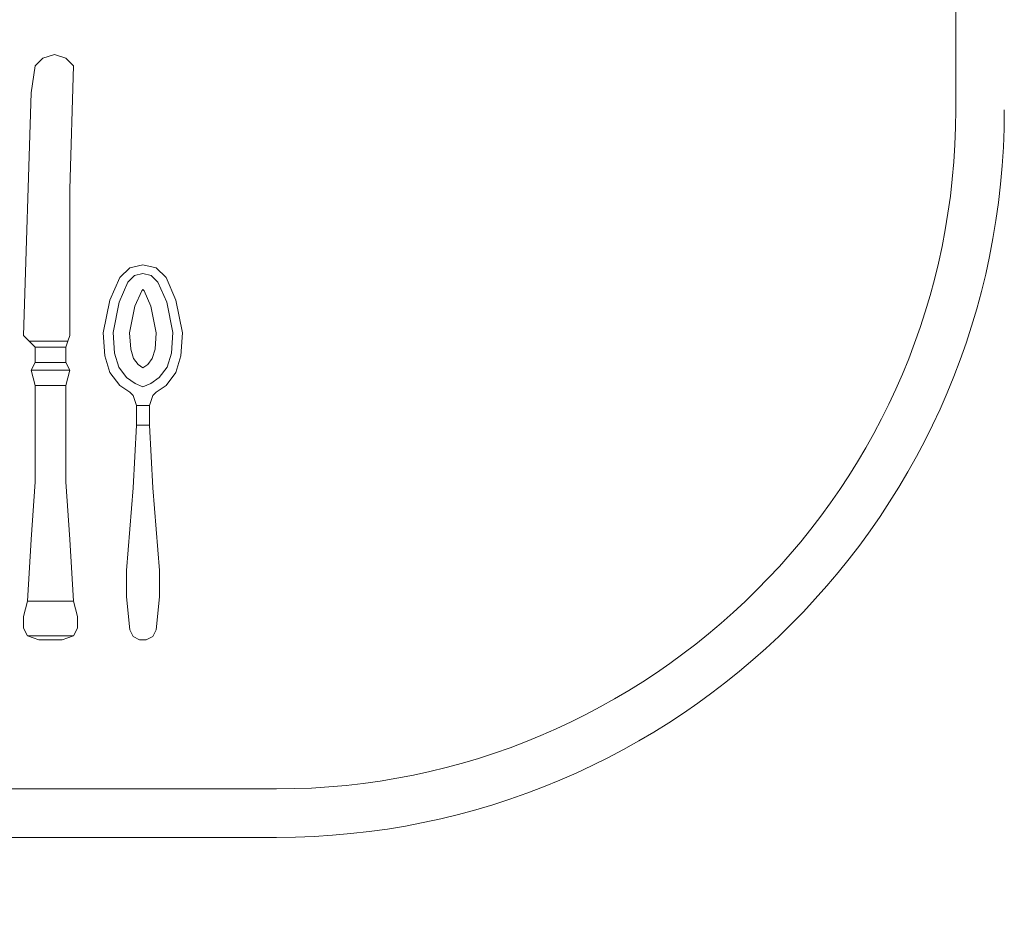
# Model space of a CAD drawing. Units: inches. Extents: x 375 to 1122, y 27 to 1069.
# Tile 105 of 155: x 731.28 to 747.02, y 845.63 to 859.8. Entities that reach past the tile are written whole.
import ezdxf

# ---------------------------------------------------------------- set-up
doc = ezdxf.new("R2010")
doc.units = ezdxf.units.IN
doc.layers.add('A-ANNO-DIMS', color=2, linetype='Continuous', lineweight=18)
doc.layers.add('Furniture', color=30, linetype='Continuous', lineweight=18)
doc.styles.get("Standard").update_dxf_attribs({"font": 'arial.ttf'})
doc.dimstyles.new('ISO-25', dxfattribs={"dimtxt": 12, "dimasz": 2.5, "dimexe": 1.5, "dimexo": 1.5, "dimtad": 1, "dimdec": 1, "dimlunit": 3, "dimtxsty": 'Standard', "dimblk": 'ARCHTICK', "dimcen": 2.5, "dimadec": 0, "dimazin": 0, "dimtfac": 1, "dimtdec": 1, "dimtmove": 0, "dimatfit": 3, "dimfxl": 1.5, "dimfxlon": 1, "dimarcsym": 0})

# ---------------------------------------------------------------- blocks, each defined once
blk = doc.blocks.new('A$C403C54AD')
for p, q in [((0.83575, 1.53256, -0.0006), (1.99923, 1.53256, -0.0006)), ((2.27071, 1.26108, -0.0006), (2.27071, 0.79569, -0.0006)), ((2.2901, 1.26108, -0.0006), (2.2901, 0.79569, -0.0006))]:
    blk.add_line(p, q)
for radius in [0.29087, 0.27148]:
    blk.add_arc((1.99923, 1.26108, -0.0006), radius, 0, 90)
for points, invisible_edges in [([(2.0754, 1.22086, -0.05249), (2.0762, 1.21716, -0.05501), (2.06818, 1.21365, -0.0533), (2.06633, 1.2169, -0.05066)], 5), ([(2.0754, 1.22086, -0.05117), (2.0762, 1.21716, -0.05369), (2.06818, 1.21365, -0.05198), (2.06633, 1.2169, -0.04934)], 5), ([(2.08833, 1.21962, -0.05699), (2.08844, 1.2235, -0.05453), (2.0754, 1.22086, -0.05249), (2.0762, 1.21716, -0.05501)], 5), ([(2.08833, 1.21962, -0.05567), (2.08844, 1.2235, -0.05321), (2.0754, 1.22086, -0.05117), (2.0762, 1.21716, -0.05369)], 5), ([(2.09764, 1.22284, -0.05408), (2.09658, 1.21902, -0.05656), (2.08833, 1.21962, -0.05567), (2.08844, 1.2235, -0.05321)], 5), ([(2.09764, 1.22284, -0.0554), (2.09658, 1.21902, -0.05788), (2.08833, 1.21962, -0.05699), (2.08844, 1.2235, -0.05453)], 5), ([(2.1021, 1.21736, -0.05707), (2.10425, 1.22086, -0.05448), (2.09764, 1.22284, -0.05408), (2.09658, 1.21902, -0.05656)], 5), ([(2.1021, 1.21736, -0.05839), (2.10425, 1.22086, -0.0558), (2.09764, 1.22284, -0.0554), (2.09658, 1.21902, -0.05788)], 5), ([(2.10951, 1.2169, -0.05628), (2.10632, 1.21421, -0.05856), (2.1021, 1.21736, -0.05839), (2.10425, 1.22086, -0.0558)], 5), ([(2.10951, 1.2169, -0.05496), (2.10632, 1.21421, -0.05724), (2.1021, 1.21736, -0.05707), (2.10425, 1.22086, -0.05448)], 5), ([(2.06818, 1.21365, -0.0533), (2.06633, 1.2169, -0.05066), (2.06249, 1.21294, -0.04957), (2.06555, 1.21097, -0.05274)], 5), ([(2.06818, 1.21365, -0.05198), (2.06633, 1.2169, -0.04934), (2.06249, 1.21294, -0.04825), (2.06555, 1.21097, -0.05142)], 5), ([(2.06818, 1.21365, -0.0533), (2.07156, 1.2081, -0.05619), (2.07778, 1.21084, -0.05782), (2.0762, 1.21716, -0.05501)], 5), ([(2.06818, 1.21365, -0.05198), (2.07156, 1.2081, -0.05487), (2.07778, 1.21084, -0.0565), (2.0762, 1.21716, -0.05369)], 5), ([(2.07778, 1.21084, -0.0565), (2.0762, 1.21716, -0.05369), (2.08833, 1.21962, -0.05567), (2.08839, 1.21299, -0.05821)], 5), ([(2.07778, 1.21084, -0.05782), (2.0762, 1.21716, -0.05501), (2.08833, 1.21962, -0.05699), (2.08839, 1.21299, -0.05953)], 5), ([(2.08833, 1.21962, -0.05699), (2.08839, 1.21299, -0.05953), (2.095, 1.21251, -0.06048), (2.09658, 1.21902, -0.05788)], 5), ([(2.08833, 1.21962, -0.05567), (2.08839, 1.21299, -0.05821), (2.095, 1.21251, -0.05916), (2.09658, 1.21902, -0.05656)], 5), ([(2.095, 1.21251, -0.06048), (2.09658, 1.21902, -0.05788), (2.1021, 1.21736, -0.05839), (2.09872, 1.2114, -0.06071)], 5), ([(2.095, 1.21251, -0.05916), (2.09658, 1.21902, -0.05656), (2.1021, 1.21736, -0.05707), (2.09872, 1.2114, -0.05939)], 5), ([(2.1021, 1.21736, -0.05839), (2.09872, 1.2114, -0.06071), (2.1011, 1.20963, -0.06081), (2.10632, 1.21421, -0.05856)], 5), ([(2.1021, 1.21736, -0.05707), (2.09872, 1.2114, -0.05939), (2.1011, 1.20963, -0.05949), (2.10632, 1.21421, -0.05724)], 5), ([(2.10861, 1.2108, -0.05857), (2.11212, 1.21294, -0.05749), (2.10951, 1.2169, -0.05628), (2.10632, 1.21421, -0.05856)], 5), ([(2.10861, 1.2108, -0.05725), (2.11212, 1.21294, -0.05534), (2.10951, 1.2169, -0.05496), (2.10632, 1.21421, -0.05724)], 5), ([(2.06249, 1.21294, -0.04957), (2.06555, 1.21097, -0.05274), (2.06475, 1.20767, -0.05255), (2.06119, 1.20767, -0.04938)], 5), ([(2.06249, 1.21294, -0.04825), (2.06555, 1.21097, -0.05142), (2.06475, 1.20767, -0.05124), (2.06119, 1.20767, -0.04806)], 5), ([(2.07156, 1.2081, -0.05487), (2.06555, 1.21097, -0.05142), (2.06818, 1.21365, -0.05198), (2.07156, 1.2081, -0.05487)], 5), ([(2.07156, 1.2081, -0.05619), (2.06555, 1.21097, -0.05274), (2.06818, 1.21365, -0.0533), (2.07156, 1.2081, -0.05619)], 5), ([(2.07778, 1.21084, -0.0565), (2.07778, 1.20449, -0.0565), (2.08839, 1.20234, -0.05821), (2.08839, 1.21299, -0.05821)], 5), ([(2.07778, 1.21084, -0.05782), (2.07778, 1.20449, -0.05782), (2.08839, 1.20234, -0.05953), (2.08839, 1.21299, -0.05953)], 5), ([(2.08839, 1.20234, -0.05953), (2.08839, 1.21299, -0.05953), (2.095, 1.21251, -0.06048), (2.095, 1.20282, -0.06048)], 5), ([(2.08839, 1.20234, -0.05821), (2.08839, 1.21299, -0.05821), (2.095, 1.21251, -0.05916), (2.095, 1.20282, -0.05916)], 5), ([(2.095, 1.21251, -0.06048), (2.095, 1.20282, -0.06048), (2.09872, 1.20393, -0.06071), (2.09872, 1.2114, -0.06071)], 5), ([(2.095, 1.21251, -0.05916), (2.095, 1.20282, -0.05916), (2.09872, 1.20393, -0.05939), (2.09872, 1.2114, -0.05939)], 5), ([(2.1011, 1.20963, -0.06081), (2.10632, 1.21421, -0.05856), (2.10861, 1.2108, -0.05857), (2.10244, 1.20767, -0.06061)], 5), ([(2.1011, 1.20963, -0.05949), (2.10632, 1.21421, -0.05724), (2.10861, 1.2108, -0.05725), (2.10244, 1.20767, -0.05929)], 5), ([(2.11212, 1.21294, -0.05749), (2.11212, 1.20767, -0.05749), (2.10997, 1.20767, -0.05839), (2.10861, 1.2108, -0.05857)], 11), ([(2.11212, 1.21294, -0.05534), (2.11212, 1.20767, -0.05534), (2.10997, 1.20767, -0.05707), (2.10861, 1.2108, -0.05725)], 11), ([(2.11345, 1.20371, -0.0546), (2.11345, 1.21162, -0.0546), (2.11212, 1.21294, -0.05534), (2.11212, 1.20239, -0.05534)], 5), ([(2.11345, 1.20371, -0.05669), (2.11345, 1.21162, -0.05669), (2.11212, 1.21294, -0.05749), (2.11212, 1.20239, -0.05749)], 5), ([(2.11345, 1.21162, -0.05669), (2.11345, 1.21162, -0.0546), (2.11212, 1.21294, -0.05534), (2.11212, 1.21294, -0.05749)], 1), ([(2.18338, 1.20107, -0.06063), (2.18338, 1.21426, -0.06063), (2.1504, 1.21162, -0.05725), (2.1504, 1.20371, -0.05725)], 5), ([(2.18338, 1.21426, -0.06063), (2.18338, 1.21426, -0.05666), (2.1504, 1.21162, -0.05462), (2.1504, 1.21162, -0.05725)], 4), ([(2.18338, 1.20107, -0.05666), (2.18338, 1.21426, -0.05666), (2.1504, 1.21162, -0.05462), (2.1504, 1.20371, -0.05462)], 5), ([(2.19393, 1.21426, -0.05694), (2.19393, 1.20107, -0.05694), (2.18338, 1.20107, -0.05666), (2.18338, 1.21426, -0.05666)], 5), ([(2.19393, 1.21426, -0.06091), (2.19393, 1.20107, -0.06091), (2.18338, 1.20107, -0.06063), (2.18338, 1.21426, -0.06063)], 5), ([(2.20713, 1.20239, -0.05691), (2.20713, 1.21294, -0.05691), (2.19393, 1.21426, -0.05694), (2.19393, 1.20107, -0.05694)], 5), ([(2.20713, 1.20239, -0.06088), (2.20713, 1.21294, -0.06088), (2.19393, 1.21426, -0.06091), (2.19393, 1.20107, -0.06091)], 5), ([(2.20976, 1.21162, -0.0567), (2.20976, 1.20371, -0.0567), (2.20713, 1.20239, -0.05691), (2.20713, 1.21294, -0.05691)], 5), ([(2.20976, 1.21162, -0.06067), (2.20976, 1.20371, -0.06067), (2.20713, 1.20239, -0.06088), (2.20713, 1.21294, -0.06088)], 5), ([(2.06475, 1.20767, -0.05124), (2.07114, 1.20767, -0.05473), (2.07156, 1.2081, -0.05487), (2.06555, 1.21097, -0.05142)], 5), ([(2.06475, 1.20767, -0.05255), (2.07114, 1.20767, -0.05605), (2.07156, 1.2081, -0.05619), (2.06555, 1.21097, -0.05274)], 5), ([(2.07156, 1.20723, -0.05619), (2.07156, 1.2081, -0.05619), (2.07778, 1.21084, -0.05782), (2.07778, 1.20449, -0.05782)], 5), ([(2.07156, 1.20723, -0.05487), (2.07156, 1.2081, -0.05487), (2.07778, 1.21084, -0.0565), (2.07778, 1.20449, -0.0565)], 5), ([(2.09872, 1.20393, -0.06071), (2.09872, 1.2114, -0.06071), (2.1011, 1.20963, -0.06081), (2.1011, 1.2057, -0.06081)], 5), ([(2.09872, 1.20393, -0.05939), (2.09872, 1.2114, -0.05939), (2.1011, 1.20963, -0.05949), (2.1011, 1.2057, -0.05949)], 5), ([(2.1011, 1.20963, -0.06081), (2.1011, 1.2057, -0.06081), (2.10244, 1.20767, -0.06061)], 1), ([(2.1011, 1.20963, -0.05949), (2.1011, 1.2057, -0.05949), (2.10244, 1.20767, -0.05929)], 1), ([(2.10861, 1.2108, -0.05857), (2.10244, 1.20767, -0.06061), (2.10244, 1.20767, -0.06061), (2.10997, 1.20767, -0.05839)], 5), ([(2.10861, 1.2108, -0.05725), (2.10244, 1.20767, -0.05929), (2.10244, 1.20767, -0.05929), (2.10997, 1.20767, -0.05707)], 5), ([(2.11741, 1.2103, -0.05275), (2.11741, 1.20503, -0.05275), (2.11345, 1.20371, -0.0546), (2.11345, 1.21162, -0.0546)], 4), ([(2.11741, 1.2103, -0.05275), (2.11741, 1.2103, -0.05497), (2.11345, 1.21162, -0.05669), (2.11345, 1.21162, -0.0546)], 5), ([(2.11741, 1.2103, -0.05497), (2.11741, 1.20503, -0.05497), (2.11345, 1.20371, -0.05669), (2.11345, 1.21162, -0.05669)], 4), ([(2.12533, 1.2103, -0.05434), (2.12533, 1.2103, -0.05212), (2.11741, 1.2103, -0.05275), (2.11741, 1.2103, -0.05497)], 5), ([(2.1504, 1.21162, -0.05462), (2.1504, 1.20371, -0.05462), (2.12533, 1.20503, -0.05212), (2.12533, 1.2103, -0.05212)], 1), ([(2.1504, 1.21162, -0.05462), (2.1504, 1.21162, -0.05725), (2.12533, 1.2103, -0.05434), (2.12533, 1.2103, -0.05212)], 5), ([(2.1504, 1.21162, -0.05725), (2.1504, 1.20371, -0.05725), (2.12533, 1.20503, -0.05434), (2.12533, 1.2103, -0.05434)], 1), ([(2.21108, 1.20635, -0.05684), (2.21108, 1.20898, -0.05684), (2.20976, 1.21162, -0.0567), (2.20976, 1.20371, -0.0567)], 4), ([(2.21108, 1.20635, -0.06038), (2.21108, 1.20898, -0.06038), (2.20976, 1.21162, -0.06067), (2.20976, 1.20371, -0.06067)], 4), ([(2.06249, 1.20239, -0.04957), (2.06555, 1.20436, -0.05274), (2.06475, 1.20767, -0.05255), (2.06119, 1.20767, -0.04938)], 5), ([(2.06249, 1.20239, -0.04825), (2.06555, 1.20436, -0.05142), (2.06475, 1.20767, -0.05124), (2.06119, 1.20767, -0.04806)], 5), ([(2.06818, 1.20168, -0.0533), (2.06633, 1.19843, -0.05066), (2.06249, 1.20239, -0.04957), (2.06555, 1.20436, -0.05274)], 5), ([(2.06818, 1.20168, -0.05198), (2.06633, 1.19843, -0.04934), (2.06249, 1.20239, -0.04825), (2.06555, 1.20436, -0.05142)], 5), ([(2.06475, 1.20767, -0.05124), (2.07114, 1.20767, -0.05473), (2.07156, 1.20723, -0.05487), (2.06555, 1.20436, -0.05142)], 5), ([(2.06475, 1.20767, -0.05255), (2.07114, 1.20767, -0.05605), (2.07156, 1.20723, -0.05619), (2.06555, 1.20436, -0.05274)], 5), ([(2.07156, 1.20723, -0.05487), (2.06555, 1.20436, -0.05142), (2.06818, 1.20168, -0.05198), (2.07156, 1.20723, -0.05487)], 5), ([(2.07156, 1.20723, -0.05619), (2.06555, 1.20436, -0.05274), (2.06818, 1.20168, -0.0533), (2.07156, 1.20723, -0.05619)], 5), ([(2.06818, 1.20168, -0.0533), (2.07156, 1.20723, -0.05619), (2.07778, 1.20449, -0.05782), (2.0762, 1.19817, -0.05501)], 5), ([(2.06818, 1.20168, -0.05198), (2.07156, 1.20723, -0.05487), (2.07778, 1.20449, -0.0565), (2.0762, 1.19817, -0.05369)], 5), ([(2.07114, 1.20767, -0.05473), (2.07156, 1.2081, -0.05487), (2.07156, 1.20723, -0.05487), (2.07114, 1.20767, -0.05473)], 2), ([(2.07114, 1.20767, -0.05605), (2.07156, 1.2081, -0.05619), (2.07156, 1.20723, -0.05619), (2.07114, 1.20767, -0.05605)], 2), ([(2.07778, 1.20449, -0.0565), (2.0762, 1.19817, -0.05369), (2.08833, 1.19571, -0.05567), (2.08839, 1.20234, -0.05821)], 5), ([(2.07778, 1.20449, -0.05782), (2.0762, 1.19817, -0.05501), (2.08833, 1.19571, -0.05699), (2.08839, 1.20234, -0.05953)], 5), ([(2.1021, 1.19797, -0.05839), (2.09872, 1.20393, -0.06071), (2.1011, 1.2057, -0.06081), (2.10632, 1.20112, -0.05856)], 5), ([(2.1021, 1.19797, -0.05707), (2.09872, 1.20393, -0.05939), (2.1011, 1.2057, -0.05949), (2.10632, 1.20112, -0.05724)], 5), ([(2.1011, 1.2057, -0.06081), (2.10632, 1.20112, -0.05856), (2.10861, 1.20453, -0.05857), (2.10244, 1.20767, -0.06061)], 5), ([(2.1011, 1.2057, -0.05949), (2.10632, 1.20112, -0.05724), (2.10861, 1.20453, -0.05725), (2.10244, 1.20767, -0.05929)], 5), ([(2.10861, 1.20453, -0.05857), (2.10244, 1.20767, -0.06061), (2.10244, 1.20767, -0.06061), (2.10997, 1.20767, -0.05839)], 5), ([(2.10861, 1.20453, -0.05725), (2.10244, 1.20767, -0.05929), (2.10244, 1.20767, -0.05929), (2.10997, 1.20767, -0.05707)], 5), ([(2.10861, 1.20453, -0.05725), (2.11212, 1.20239, -0.05534), (2.10951, 1.19843, -0.05496), (2.10632, 1.20112, -0.05724)], 5), ([(2.11212, 1.20239, -0.05749), (2.11212, 1.20767, -0.05749), (2.10997, 1.20767, -0.05839), (2.10861, 1.20453, -0.05857)], 11), ([(2.11212, 1.20239, -0.05534), (2.11212, 1.20767, -0.05534), (2.10997, 1.20767, -0.05707), (2.10861, 1.20453, -0.05725)], 11), ([(2.11741, 1.20503, -0.05497), (2.11741, 1.20503, -0.05275), (2.11345, 1.20371, -0.0546), (2.11345, 1.20371, -0.05669)], 5), ([(2.11741, 1.20503, -0.05497), (2.11741, 1.20503, -0.05275), (2.12533, 1.20503, -0.05212), (2.12533, 1.20503, -0.05434)], 5), ([(2.12533, 1.20503, -0.05212), (2.12533, 1.20503, -0.05434), (2.1504, 1.20371, -0.05725), (2.1504, 1.20371, -0.05462)], 5), ([(2.0754, 1.19447, -0.05249), (2.0762, 1.19817, -0.05501), (2.06818, 1.20168, -0.0533), (2.06633, 1.19843, -0.05066)], 5), ([(2.0754, 1.19447, -0.05117), (2.0762, 1.19817, -0.05369), (2.06818, 1.20168, -0.05198), (2.06633, 1.19843, -0.04934)], 5), ([(2.08833, 1.19571, -0.05699), (2.08839, 1.20234, -0.05953), (2.095, 1.20282, -0.06048), (2.09658, 1.19631, -0.05788)], 5), ([(2.08833, 1.19571, -0.05567), (2.08839, 1.20234, -0.05821), (2.095, 1.20282, -0.05916), (2.09658, 1.19631, -0.05656)], 5), ([(2.095, 1.20282, -0.05916), (2.09658, 1.19631, -0.05656), (2.1021, 1.19797, -0.05707), (2.09872, 1.20393, -0.05939)], 5), ([(2.10951, 1.19843, -0.05628), (2.10632, 1.20112, -0.05856), (2.1021, 1.19797, -0.05839), (2.10425, 1.19447, -0.0558)], 5), ([(2.10951, 1.19843, -0.05496), (2.10632, 1.20112, -0.05724), (2.1021, 1.19797, -0.05707), (2.10425, 1.19447, -0.05448)], 5), ([(2.11345, 1.20371, -0.0546), (2.11345, 1.20371, -0.05669), (2.11212, 1.20239, -0.05749), (2.11212, 1.20239, -0.05534)], 1), ([(2.1504, 1.20371, -0.05725), (2.1504, 1.20371, -0.05462), (2.18338, 1.20107, -0.05666), (2.18338, 1.20107, -0.06063)], 1), ([(2.08833, 1.19571, -0.05699), (2.08844, 1.19183, -0.05453), (2.0754, 1.19447, -0.05249), (2.0762, 1.19817, -0.05501)], 5), ([(2.08833, 1.19571, -0.05567), (2.08844, 1.19183, -0.05321), (2.0754, 1.19447, -0.05117), (2.0762, 1.19817, -0.05369)], 5), ([(2.1021, 1.19797, -0.05707), (2.10425, 1.19447, -0.05448), (2.09764, 1.19249, -0.05408), (2.09658, 1.19631, -0.05656)], 5), ([(2.1021, 1.19797, -0.05839), (2.10425, 1.19447, -0.0558), (2.09764, 1.19249, -0.0554), (2.09658, 1.19631, -0.05788)], 5), ([(2.09764, 1.19249, -0.05408), (2.09658, 1.19631, -0.05656), (2.08833, 1.19571, -0.05567), (2.08844, 1.19183, -0.05321)], 5), ([(2.09764, 1.19249, -0.0554), (2.09658, 1.19631, -0.05788), (2.08833, 1.19571, -0.05699), (2.08844, 1.19183, -0.05453)], 5), ([(2.19569, 1.17996, -0.05014), (2.19569, 1.16149, -0.05014), (2.20185, 1.15995, -0.0486), (2.20185, 1.1815, -0.0486)], 4), ([(2.19569, 1.17996, -0.05938), (2.19569, 1.16149, -0.05938), (2.20185, 1.15995, -0.06091), (2.20185, 1.1815, -0.06091)], 4), ([(2.20185, 1.15995, -0.0486), (2.20185, 1.1815, -0.0486), (2.20647, 1.1815, -0.05014), (2.20647, 1.15995, -0.05014)], 5), ([(2.20185, 1.15995, -0.06091), (2.20185, 1.1815, -0.06091), (2.20647, 1.1815, -0.05938), (2.20647, 1.15995, -0.05938)], 5), ([(2.20647, 1.1815, -0.05014), (2.20647, 1.15995, -0.05014), (2.20954, 1.16149, -0.05168), (2.20954, 1.17996, -0.05168)], 1), ([(2.20647, 1.1815, -0.05938), (2.20647, 1.15995, -0.05938), (2.20954, 1.16149, -0.05784), (2.20954, 1.17996, -0.05784)], 1), ([(1.97713, 1.17226, -0.05399), (1.97713, 1.17226, -0.05399), (1.97867, 1.17688, -0.05399), (1.97867, 1.16765, -0.05399)], 4), ([(1.97713, 1.17226, -0.05553), (1.97713, 1.17226, -0.05553), (1.97867, 1.17688, -0.05553), (1.97867, 1.16765, -0.05553)], 4), ([(1.97867, 1.17688, -0.05553), (1.97867, 1.17688, -0.05399), (1.97713, 1.17226, -0.05399), (1.97713, 1.17226, -0.05553)], 1), ([(1.97867, 1.17688, -0.05399), (1.97867, 1.16765, -0.05399), (1.98174, 1.16457, -0.05399), (1.98174, 1.17996, -0.05399)], 5), ([(1.97867, 1.17688, -0.05553), (1.97867, 1.16765, -0.05553), (1.98174, 1.16457, -0.05553), (1.98174, 1.17996, -0.05553)], 5), ([(1.98174, 1.17996, -0.05399), (1.98174, 1.17996, -0.05553), (1.97867, 1.17688, -0.05553), (1.97867, 1.17688, -0.05399)], 5), ([(1.98174, 1.16457, -0.05399), (1.98174, 1.17996, -0.05399), (2.031, 1.17842, -0.05399), (1.99252, 1.16303, -0.05399)], 5), ([(1.98174, 1.16457, -0.05553), (1.98174, 1.17996, -0.05553), (2.031, 1.17842, -0.05553), (1.99252, 1.16303, -0.05553)], 5), ([(2.031, 1.17842, -0.05553), (2.031, 1.17842, -0.05399), (1.98174, 1.17996, -0.05399), (1.98174, 1.17996, -0.05553)], 5), ([(2.031, 1.17842, -0.05399), (1.99252, 1.16303, -0.05399), (2.08949, 1.15995, -0.05399), (2.08949, 1.17842, -0.05399)], 5), ([(2.031, 1.17842, -0.05553), (1.99252, 1.16303, -0.05553), (2.08949, 1.15995, -0.05553), (2.08949, 1.17842, -0.05553)], 5), ([(2.08949, 1.17842, -0.05399), (2.08949, 1.17842, -0.05553), (2.031, 1.17842, -0.05553), (2.031, 1.17842, -0.05399)], 5), ([(2.08949, 1.15995, -0.05399), (2.08949, 1.17842, -0.05399), (2.0918, 1.17765, -0.05322), (2.0918, 1.16226, -0.05322)], 1), ([(2.08949, 1.15995, -0.05553), (2.08949, 1.17842, -0.05553), (2.0918, 1.17765, -0.0563), (2.0918, 1.16226, -0.0563)], 1), ([(2.0918, 1.17765, -0.0563), (2.0918, 1.17765, -0.05322), (2.08949, 1.17842, -0.05399), (2.08949, 1.17842, -0.05553)], 5), ([(2.0941, 1.17688, -0.05014), (2.0941, 1.17688, -0.05938), (2.0918, 1.17765, -0.0563), (2.0918, 1.17765, -0.05322)], 5), ([(2.10026, 1.17688, -0.05938), (2.10026, 1.17688, -0.05014), (2.0941, 1.17688, -0.05014), (2.0941, 1.17688, -0.05938)], 4), ([(2.1095, 1.16457, -0.05014), (2.1095, 1.17688, -0.05014), (2.14798, 1.17688, -0.0486), (2.14798, 1.16457, -0.0486)], 4), ([(2.1095, 1.16457, -0.05938), (2.1095, 1.17688, -0.05938), (2.14798, 1.17688, -0.06091), (2.14798, 1.16457, -0.06091)], 4), ([(2.14798, 1.17688, -0.0486), (2.14798, 1.16457, -0.0486), (2.17106, 1.16303, -0.0486), (2.17106, 1.17842, -0.0486)], 5), ([(2.14798, 1.17688, -0.06091), (2.14798, 1.16457, -0.06091), (2.17106, 1.16303, -0.06091), (2.17106, 1.17842, -0.06091)], 5), ([(2.17106, 1.16303, -0.0486), (2.17106, 1.17842, -0.0486), (2.19569, 1.17996, -0.05014), (2.19569, 1.16149, -0.05014)], 1), ([(2.17106, 1.16303, -0.06091), (2.17106, 1.17842, -0.06091), (2.19569, 1.17996, -0.05938), (2.19569, 1.16149, -0.05938)], 1), ([(1.97713, 1.17226, -0.05399), (1.97713, 1.17226, -0.05553), (1.97867, 1.16765, -0.05553), (1.97867, 1.16765, -0.05399)], 4), ([(1.97867, 1.16765, -0.05553), (1.97867, 1.16765, -0.05399), (1.98174, 1.16457, -0.05399), (1.98174, 1.16457, -0.05553)], 5), ([(1.98174, 1.16457, -0.05399), (1.98174, 1.16457, -0.05553), (1.99252, 1.16303, -0.05553), (1.99252, 1.16303, -0.05399)], 5), ([(1.99252, 1.16303, -0.05553), (1.99252, 1.16303, -0.05399), (2.08949, 1.15995, -0.05399), (2.08949, 1.15995, -0.05553)], 5), ([(2.08949, 1.15995, -0.05553), (2.08949, 1.15995, -0.05399), (2.0918, 1.16226, -0.05322), (2.0918, 1.16226, -0.0563)], 5), ([(2.0918, 1.16226, -0.05322), (2.0918, 1.16226, -0.0563), (2.0941, 1.16457, -0.05938), (2.0941, 1.16457, -0.05014)], 5), ([(2.0941, 1.16457, -0.05938), (2.0941, 1.16457, -0.05014), (2.10026, 1.16457, -0.05014), (2.10026, 1.16457, -0.05938)], 1)]:
    blk.add_3dface(points, dxfattribs=dict(invisible_edges=invisible_edges))
for points in [[(2.0754, 1.22086, -0.05117), (2.0754, 1.22086, -0.05249), (2.06633, 1.2169, -0.05066), (2.06633, 1.2169, -0.04934)], [(2.08844, 1.2235, -0.05453), (2.08844, 1.2235, -0.05321), (2.0754, 1.22086, -0.05117), (2.0754, 1.22086, -0.05249)], [(2.09764, 1.22284, -0.05408), (2.09764, 1.22284, -0.0554), (2.08844, 1.2235, -0.05453), (2.08844, 1.2235, -0.05321)], [(2.10425, 1.22086, -0.0558), (2.10425, 1.22086, -0.05448), (2.09764, 1.22284, -0.05408), (2.09764, 1.22284, -0.0554)], [(2.10951, 1.2169, -0.05496), (2.10951, 1.2169, -0.05628), (2.10425, 1.22086, -0.0558), (2.10425, 1.22086, -0.05448)], [(2.06633, 1.2169, -0.05066), (2.06633, 1.2169, -0.04934), (2.06249, 1.21294, -0.04825), (2.06249, 1.21294, -0.04957)], [(2.11212, 1.21294, -0.05749), (2.11212, 1.21294, -0.05534), (2.10951, 1.2169, -0.05496), (2.10951, 1.2169, -0.05628)], [(2.06249, 1.21294, -0.04825), (2.06249, 1.21294, -0.04957), (2.06119, 1.20767, -0.04938), (2.06119, 1.20767, -0.04806)], [(2.19393, 1.21426, -0.05694), (2.19393, 1.21426, -0.06091), (2.18338, 1.21426, -0.06063), (2.18338, 1.21426, -0.05666)], [(2.20713, 1.21294, -0.06088), (2.20713, 1.21294, -0.05691), (2.19393, 1.21426, -0.05694), (2.19393, 1.21426, -0.06091)], [(2.20976, 1.21162, -0.0567), (2.20976, 1.21162, -0.06067), (2.20713, 1.21294, -0.06088), (2.20713, 1.21294, -0.05691)], [(2.12533, 1.20503, -0.05434), (2.12533, 1.2103, -0.05434), (2.11741, 1.2103, -0.05497), (2.11741, 1.20503, -0.05497)], [(2.12533, 1.20503, -0.05212), (2.12533, 1.2103, -0.05212), (2.11741, 1.2103, -0.05275), (2.11741, 1.20503, -0.05275)], [(2.21108, 1.20898, -0.06038), (2.21108, 1.20898, -0.05684), (2.20976, 1.21162, -0.0567), (2.20976, 1.21162, -0.06067)], [(2.21108, 1.20635, -0.05684), (2.21108, 1.20635, -0.06038), (2.21108, 1.20898, -0.06038), (2.21108, 1.20898, -0.05684)], [(2.06119, 1.20767, -0.04938), (2.06119, 1.20767, -0.04806), (2.06249, 1.20239, -0.04825), (2.06249, 1.20239, -0.04957)], [(2.20976, 1.20371, -0.06067), (2.20976, 1.20371, -0.0567), (2.21108, 1.20635, -0.05684), (2.21108, 1.20635, -0.06038)], [(2.06249, 1.20239, -0.04825), (2.06249, 1.20239, -0.04957), (2.06633, 1.19843, -0.05066), (2.06633, 1.19843, -0.04934)], [(2.10951, 1.19843, -0.05628), (2.10951, 1.19843, -0.05496), (2.11212, 1.20239, -0.05534), (2.11212, 1.20239, -0.05749)], [(2.18338, 1.20107, -0.05666), (2.18338, 1.20107, -0.06063), (2.19393, 1.20107, -0.06091), (2.19393, 1.20107, -0.05694)], [(2.19393, 1.20107, -0.06091), (2.19393, 1.20107, -0.05694), (2.20713, 1.20239, -0.05691), (2.20713, 1.20239, -0.06088)], [(2.20713, 1.20239, -0.05691), (2.20713, 1.20239, -0.06088), (2.20976, 1.20371, -0.06067), (2.20976, 1.20371, -0.0567)], [(2.06633, 1.19843, -0.05066), (2.06633, 1.19843, -0.04934), (2.0754, 1.19447, -0.05117), (2.0754, 1.19447, -0.05249)], [(2.10425, 1.19447, -0.05448), (2.10425, 1.19447, -0.0558), (2.10951, 1.19843, -0.05628), (2.10951, 1.19843, -0.05496)], [(2.0754, 1.19447, -0.05117), (2.0754, 1.19447, -0.05249), (2.08844, 1.19183, -0.05453), (2.08844, 1.19183, -0.05321)], [(2.08844, 1.19183, -0.05453), (2.08844, 1.19183, -0.05321), (2.09764, 1.19249, -0.05408), (2.09764, 1.19249, -0.0554)], [(2.09764, 1.19249, -0.0554), (2.09764, 1.19249, -0.05408), (2.10425, 1.19447, -0.05448), (2.10425, 1.19447, -0.0558)], [(2.20185, 1.1815, -0.06091), (2.20185, 1.1815, -0.0486), (2.19569, 1.17996, -0.05014), (2.19569, 1.17996, -0.05938)], [(2.20647, 1.1815, -0.05014), (2.20647, 1.1815, -0.05938), (2.20185, 1.1815, -0.06091), (2.20185, 1.1815, -0.0486)], [(2.20954, 1.17996, -0.05168), (2.20954, 1.17996, -0.05784), (2.20647, 1.1815, -0.05938), (2.20647, 1.1815, -0.05014)], [(2.0918, 1.16226, -0.05322), (2.0918, 1.17765, -0.05322), (2.0941, 1.17688, -0.05014), (2.0941, 1.16457, -0.05014)], [(2.0918, 1.16226, -0.0563), (2.0918, 1.17765, -0.0563), (2.0941, 1.17688, -0.05938), (2.0941, 1.16457, -0.05938)], [(2.0941, 1.17688, -0.05014), (2.0941, 1.16457, -0.05014), (2.10026, 1.16457, -0.05014), (2.10026, 1.17688, -0.05014)], [(2.0941, 1.17688, -0.05938), (2.0941, 1.16457, -0.05938), (2.10026, 1.16457, -0.05938), (2.10026, 1.17688, -0.05938)], [(2.10026, 1.16457, -0.05014), (2.10026, 1.17688, -0.05014), (2.10334, 1.17842, -0.0486), (2.10334, 1.16303, -0.0486)], [(2.10026, 1.16457, -0.05938), (2.10026, 1.17688, -0.05938), (2.10334, 1.17842, -0.06091), (2.10334, 1.16303, -0.06091)], [(2.10334, 1.17842, -0.0486), (2.10334, 1.17842, -0.06091), (2.10026, 1.17688, -0.05938), (2.10026, 1.17688, -0.05014)], [(2.10334, 1.17842, -0.0486), (2.10334, 1.16303, -0.0486), (2.1095, 1.16457, -0.05014), (2.1095, 1.17688, -0.05014)], [(2.10334, 1.17842, -0.06091), (2.10334, 1.16303, -0.06091), (2.1095, 1.16457, -0.05938), (2.1095, 1.17688, -0.05938)], [(2.1095, 1.17688, -0.05938), (2.1095, 1.17688, -0.05014), (2.10334, 1.17842, -0.0486), (2.10334, 1.17842, -0.06091)], [(2.14798, 1.17688, -0.0486), (2.14798, 1.17688, -0.06091), (2.1095, 1.17688, -0.05938), (2.1095, 1.17688, -0.05014)], [(2.17106, 1.17842, -0.06091), (2.17106, 1.17842, -0.0486), (2.14798, 1.17688, -0.0486), (2.14798, 1.17688, -0.06091)], [(2.19569, 1.17996, -0.05014), (2.19569, 1.17996, -0.05938), (2.17106, 1.17842, -0.06091), (2.17106, 1.17842, -0.0486)], [(2.20954, 1.16149, -0.05168), (2.20954, 1.17996, -0.05168), (2.21108, 1.17534, -0.05476), (2.21108, 1.16611, -0.05476)], [(2.21108, 1.17534, -0.05476), (2.21108, 1.17534, -0.05476), (2.20954, 1.17996, -0.05168), (2.20954, 1.17996, -0.05784)], [(2.20954, 1.16149, -0.05784), (2.20954, 1.17996, -0.05784), (2.21108, 1.17534, -0.05476), (2.21108, 1.16611, -0.05476)], [(2.20954, 1.16149, -0.05168), (2.20954, 1.16149, -0.05784), (2.21108, 1.16611, -0.05476)], [(2.10026, 1.16457, -0.05014), (2.10026, 1.16457, -0.05938), (2.10334, 1.16303, -0.06091), (2.10334, 1.16303, -0.0486)], [(2.10334, 1.16303, -0.06091), (2.10334, 1.16303, -0.0486), (2.1095, 1.16457, -0.05014), (2.1095, 1.16457, -0.05938)], [(2.1095, 1.16457, -0.05014), (2.1095, 1.16457, -0.05938), (2.14798, 1.16457, -0.06091), (2.14798, 1.16457, -0.0486)], [(2.14798, 1.16457, -0.06091), (2.14798, 1.16457, -0.0486), (2.17106, 1.16303, -0.0486), (2.17106, 1.16303, -0.06091)], [(2.17106, 1.16303, -0.0486), (2.17106, 1.16303, -0.06091), (2.19569, 1.16149, -0.05938), (2.19569, 1.16149, -0.05014)], [(2.19569, 1.16149, -0.05938), (2.19569, 1.16149, -0.05014), (2.20185, 1.15995, -0.0486), (2.20185, 1.15995, -0.06091)], [(2.20647, 1.15995, -0.05938), (2.20647, 1.15995, -0.05014), (2.20954, 1.16149, -0.05168), (2.20954, 1.16149, -0.05784)], [(2.20185, 1.15995, -0.0486), (2.20185, 1.15995, -0.06091), (2.20647, 1.15995, -0.05938), (2.20647, 1.15995, -0.05014)]]:
    blk.add_3dface(points)
blk = doc.blocks.new('_ArchTick')
at = {"color": 0, "linetype": 'ByBlock', "const_width": 0.15}
blk.add_lwpolyline([(-0.5, -0.5), (0.5, 0.5)], dxfattribs=at)
blk = doc.blocks.new('*D85')
at = {"layer": 'A-ANNO-DIMS', "color": 0, "lineweight": -2, "transparency": 16777216}
for p, q in [((401.507, 868.528), (398.507, 868.528)), ((400.007, 814.528), (400.007, 868.528)), ((401.507, 814.528), (398.507, 814.528))]:
    blk.add_line(p, q, dxfattribs=at)
at = {"layer": 'Defpoints', "color": 0, "transparency": 16777216}
for p in [(400.007, 868.528), (845.007, 868.528), (845.007, 814.528)]:
    blk.add_point(p, dxfattribs=at)
at = {"layer": 'A-ANNO-DIMS', "color": 0, "lineweight": -2, "transparency": 16777216, "xscale": 2.5, "yscale": 2.5, "zscale": 2.5}
for p, rotation in [((400.007, 868.528), 90), ((400.007, 814.528), 270)]:
    blk.add_blockref('_ArchTick', p, dxfattribs=dict(at, rotation=rotation))
at = {"layer": 'A-ANNO-DIMS', "color": 0, "transparency": 16777216, "insert": (393.255, 841.528), "char_height": 12, "attachment_point": 5, "rotation": 90}
blk.add_mtext('4\'-6"', dxfattribs=at)
blk = doc.blocks.new('*D88')
at = {"layer": 'A-ANNO-DIMS', "color": 0, "lineweight": -2, "transparency": 16777216}
for p, q in [((731.007, 1052.528), (731.007, 1055.528)), ((854.007, 1052.528), (854.007, 1055.528)), ((731.007, 1054.028), (854.007, 1054.028))]:
    blk.add_line(p, q, dxfattribs=at)
at = {"layer": 'Defpoints', "color": 0, "transparency": 16777216}
for p in [(854.007, 1054.028), (731.007, 502.528), (854.007, 502.528)]:
    blk.add_point(p, dxfattribs=at)
at = {"layer": 'A-ANNO-DIMS', "color": 0, "lineweight": -2, "transparency": 16777216, "xscale": 2.5, "yscale": 2.5, "zscale": 2.5, "rotation": 180}
blk.add_blockref('_ArchTick', (731.007, 1054.028), dxfattribs=at)
at = {"layer": 'A-ANNO-DIMS', "color": 0, "lineweight": -2, "transparency": 16777216, "xscale": 2.5, "yscale": 2.5, "zscale": 2.5}
blk.add_blockref('_ArchTick', (854.007, 1054.028), dxfattribs=at)
at = {"layer": 'A-ANNO-DIMS', "color": 0, "transparency": 16777216, "insert": (792.507, 1060.784), "char_height": 12, "attachment_point": 5}
blk.add_mtext('10\'-3"', dxfattribs=at)
blk = doc.blocks.new('*D91')
at = {"layer": 'A-ANNO-DIMS', "color": 0, "lineweight": -2, "transparency": 16777216}
for p, q in [((728.007, 1052.528), (728.007, 1055.528)), ((788.007, 1052.528), (788.007, 1055.528)), ((728.007, 1054.028), (788.007, 1054.028))]:
    blk.add_line(p, q, dxfattribs=at)
at = {"layer": 'Defpoints', "color": 0, "transparency": 16777216}
for p in [(788.007, 1054.028), (728.007, 774.028), (788.007, 774.028)]:
    blk.add_point(p, dxfattribs=at)
at = {"layer": 'A-ANNO-DIMS', "color": 0, "lineweight": -2, "transparency": 16777216, "xscale": 2.5, "yscale": 2.5, "zscale": 2.5, "rotation": 180}
blk.add_blockref('_ArchTick', (728.007, 1054.028), dxfattribs=at)
at = {"layer": 'A-ANNO-DIMS', "color": 0, "lineweight": -2, "transparency": 16777216, "xscale": 2.5, "yscale": 2.5, "zscale": 2.5}
blk.add_blockref('_ArchTick', (788.007, 1054.028), dxfattribs=at)
at = {"layer": 'A-ANNO-DIMS', "color": 0, "transparency": 16777216, "insert": (758.007, 1060.78), "char_height": 12, "attachment_point": 5}
blk.add_mtext('5\'-0"', dxfattribs=at)

msp = doc.modelspace()

# ---------------------------------------------------------------- block references
at = {"layer": 'Furniture', "xscale": 39.9918517141215, "yscale": 39.9918517141215, "zscale": 39.9918517141215, "rotation": 270}
msp.add_blockref('A$C403C54AD', (684.955, 938.316, 0.024), dxfattribs=at)

# ---------------------------------------------------------------- dimensions: what is measured, and where the dimension line sits
at = {"layer": 'A-ANNO-DIMS'}
for base, p1, p2, picture, middle in [((788.007, 1054.028), (728.007, 774.028), (788.007, 774.028), '*D91', (758.007, 1060.78)), ((854.007, 1054.028), (731.007, 502.528), (854.007, 502.528), '*D88', (792.507, 1060.784))]:
    dim = msp.add_linear_dim(base=base, p1=p1, p2=p2, dimstyle='ISO-25', override={"dimdec": 1, "dimlfac": 1, "dimrnd": 0, "dimzin": 1, "dimdsep": 46, "dimlunit": 4, "dimfrac": 2}, dxfattribs=at)
    dim.commit()
    dim.dimension.update_dxf_attribs({"geometry": picture, "text_midpoint": middle})
dim = msp.add_linear_dim(base=(400.007, 868.528), p1=(845.007, 814.528), p2=(845.007, 868.528), angle=90, dimstyle='ISO-25', override={"dimdec": 1, "dimlfac": 1, "dimrnd": 0, "dimzin": 1, "dimdsep": 46, "dimlunit": 4, "dimfrac": 2}, dxfattribs=at)
dim.commit()
dim.dimension.update_dxf_attribs({"geometry": '*D85', "text_midpoint": (393.255, 841.528)})

doc.saveas('drawing.dxf')
